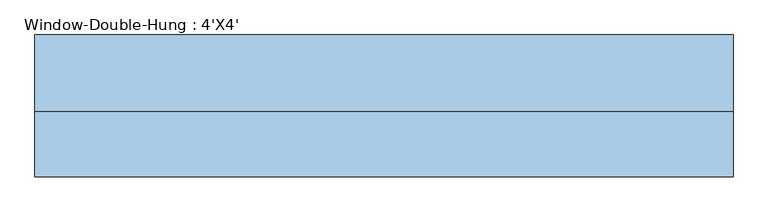
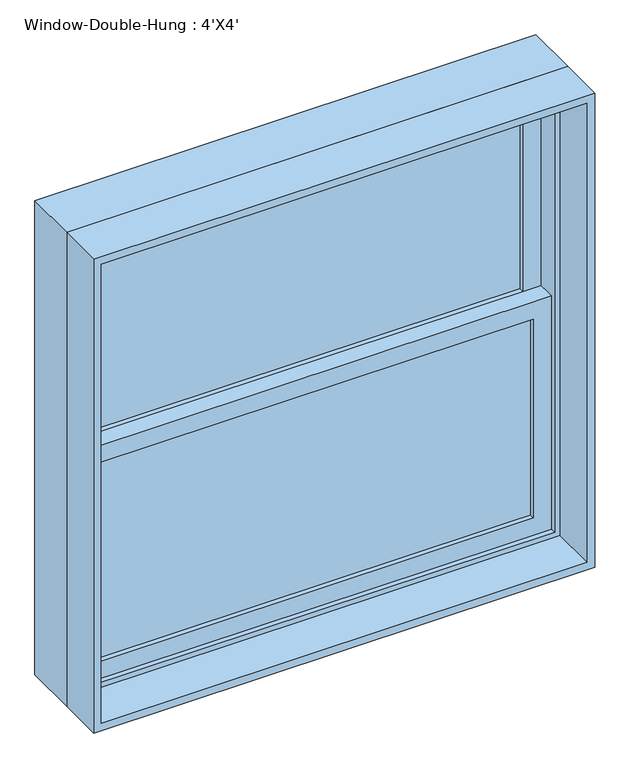
"""IFC4 building model written with IfcOpenShell, lengths in millimetres: window geometry, Window-Double-Hung : 4'X4'."""

from ifc_helpers import new_model, si_unit, frame, origin, place, context, project, spatial, polyline, outline, extrude, source, transform, mapped, element, save


def window_double_hung_4_x4_ec8efb0e(model_context):
    return source(origin(), model_context, "Body", "SweptSolid", [
        extrude(outline(polyline([(533.4, 44.45), (533.4, 38.1), (-533.4, 38.1), (-533.4, 44.45), (533.4, 44.45)])), frame((0.0, 0.0, 990.6), z_axis=(0.0, 0.0, 1.0), x_axis=(1.0, 0.0, 0.0)), (0.0, 0.0, 1.0), 511.175),
        extrude(outline(polyline([(-533.4, 31.75), (533.4, 31.75), (533.4, 25.4), (-533.4, 25.4), (-533.4, 31.75)])), frame((0.0, 0.0, 990.6), z_axis=(0.0, 0.0, 1.0), x_axis=(1.0, 0.0, 0.0)), (0.0, 0.0, 1.0), 511.175),
        extrude(outline(polyline([(533.4, 88.9), (533.4, 82.55), (-533.4, 82.55), (-533.4, 88.9), (533.4, 88.9)])), frame((0.0, 0.0, 1546.225), z_axis=(0.0, 0.0, 1.0), x_axis=(1.0, 0.0, 0.0)), (0.0, 0.0, 1.0), 511.175),
        extrude(outline(polyline([(-533.4, 76.2), (533.4, 76.2), (533.4, 69.85), (-533.4, 69.85), (-533.4, 76.2)])), frame((0.0, 0.0, 1546.225), z_axis=(0.0, 0.0, 1.0), x_axis=(1.0, 0.0, 0.0)), (0.0, 0.0, 1.0), 511.175),
        extrude(outline(polyline([(1546.225, -577.85), (946.15, -577.85), (946.15, 577.85), (1546.225, 577.85), (1546.225, -577.85)]), holes=[polyline([(1501.775, 533.4), (990.6, 533.4), (990.6, -533.4), (1501.775, -533.4), (1501.775, 533.4)])]), frame((0.0, 12.7, 0.0), z_axis=(0.0, 1.0, 0.0), x_axis=(0.0, 0.0, 1.0)), (0.0, 0.0, 1.0), 44.45),
        extrude(outline(polyline([(2101.85, -577.85), (1501.775, -577.85), (1501.775, 577.85), (2101.85, 577.85), (2101.85, -577.85)]), holes=[polyline([(2057.4, 533.4), (1546.225, 533.4), (1546.225, -533.4), (2057.4, -533.4), (2057.4, 533.4)])]), frame((0.0, 57.15, 0.0), z_axis=(0.0, 1.0, 0.0), x_axis=(0.0, 0.0, 1.0)), (0.0, 0.0, 1.0), 44.45),
        extrude(outline(polyline([(2133.6, -609.6), (914.4, -609.6), (914.4, 609.6), (2133.6, 609.6), (2133.6, -609.6)]), holes=[polyline([(2101.85, 577.85), (946.15, 577.85), (946.15, -577.85), (2101.85, -577.85), (2101.85, 577.85)])]), frame((0.0, 0.0, 0.0), z_axis=(0.0, 1.0, 0.0), x_axis=(0.0, 0.0, 1.0)), (0.0, 0.0, 1.0), 133.35),
        extrude(outline(polyline([(2133.6, 609.6), (2133.6, -609.6), (914.4, -609.6), (914.4, 609.6), (2133.6, 609.6)]), holes=[polyline([(2114.55, 590.55), (933.45, 590.55), (933.45, -590.55), (2114.55, -590.55), (2114.55, 590.55)])]), frame((0.0, -114.3, 0.0), z_axis=(0.0, 1.0, 0.0), x_axis=(0.0, 0.0, 1.0)), (0.0, 0.0, 1.0), 114.3),
    ])


if __name__ == "__main__":
    model = new_model("IFC4")
    model_context = context("Model", 3, world=origin())
    ifc_project = project(units=[si_unit("LENGTHUNIT", "METRE", prefix="MILLI")], contexts=[model_context])
    site = spatial("IfcSite", under=ifc_project)
    building = spatial("IfcBuilding", under=site)
    placement = place(None, origin())
    window_double_hung_4_x4_shape = window_double_hung_4_x4_ec8efb0e(model_context)
    element("IfcWindow", 1, ObjectType="Window-Double-Hung : 4'X4'", at=placement, inside=building, context=model_context, shape_type="MappedRepresentation", body=[
        mapped(window_double_hung_4_x4_shape, transform((0.0, 0.0, 0.0), x_axis=(1.0, 0.0, 0.0), y_axis=(0.0, 1.0, 0.0), z_axis=(0.0, 0.0, 1.0))),
    ])
    save(model, "model.ifc")

# Revit data of these elements
# Type "Window-Double-Hung : 4'X4'"
#   Type Mark = "19"
#   Fire Rating = "0.5h"
#   Construction Type Id = "DG-DR"
#   Assembly Code = "B2020100"
#   Analytic Construction = "Double glazing - domestic"
#   Wall Thickness [instance default] = 0' - 6"
#   Window Inset [instance default] = 0' - 0"
#   Visual Light Transmittance = 0.81
#   Thermal Resistance (R) = 1.8146 (h·ft²·°F)/BTU
#   Solar Heat Gain Coefficient = 0.76
#   Muntin Width = 3' - 6"
#   Muntin Height = 1' - 8 1/8"
#   Interior Wall Closure [instance default] = 0' - 1 1/2"
#   Rough Width = 4' - 0 1/2"
#   Rough Height = 4' - 0 1/2"
#   Frame Extension [instance default] = 0' - 1 1/4"
#   Exterior Wall Closure [instance default] = 0' - 0 1/2"
#   Extension Jamb [instance default] = 0' - 1 1/2"
#   Heat Transfer Coefficient (U) = 0.5511 BTU/(h·ft²·°F)
#   Height = 4' - 0"
#   Width = 4' - 0"
#   Top Muntin Visibility = yes
#   Indicator Visibility [instance default] = yes
#   Extension Jamb Visibility [instance default] = yes
#   Interior Trim Visibility [instance default] = yes
#   Exterior Trim Visibility [instance default] = yes
#   Define Thermal Properties by = 1
#   Bottom Muntin Visibility = yes
#   Muntin Pattern = Muntin Pattern_2x2 : Muntin Pattern_2x2
#   Interior Trim Material = Wood - Stained
#   Interior Trim = Trim-Window-Interior-Flat : Picture Frame
#   Exterior Trim Material = Clad - White
#   Exterior Trim = Trim-Window-Exterior-Flat : with Sill
#   Glass Panel Material = Glass
#   Exterior Frame Material = Clad - White
#   Interior Frame Material = Wood - Stained
#   Wall Closure = (empty or 0)
# Element 1 (IfcWindow, "Window-Double-Hung : 4'X4'")
#   Wall Thickness = 0' - 9"
#   Extension Jamb = 0' - 4 1/2"
#   Materials on its faces: "Wood - Stained", "Glass", "Clad - White"
# Materials
#   "Wood - Stained": class "Wood", colour RGB 224 178 126, transparency 0, Cost = 0
#   "Clad - White": class "Wood", colour RGB 242 242 238, transparency 0, Cost = 0
#   "Glass": class "Glass", colour RGB 0 128 192, transparency 0.75, Description = "Soda Lime Glass", Cost = 0
